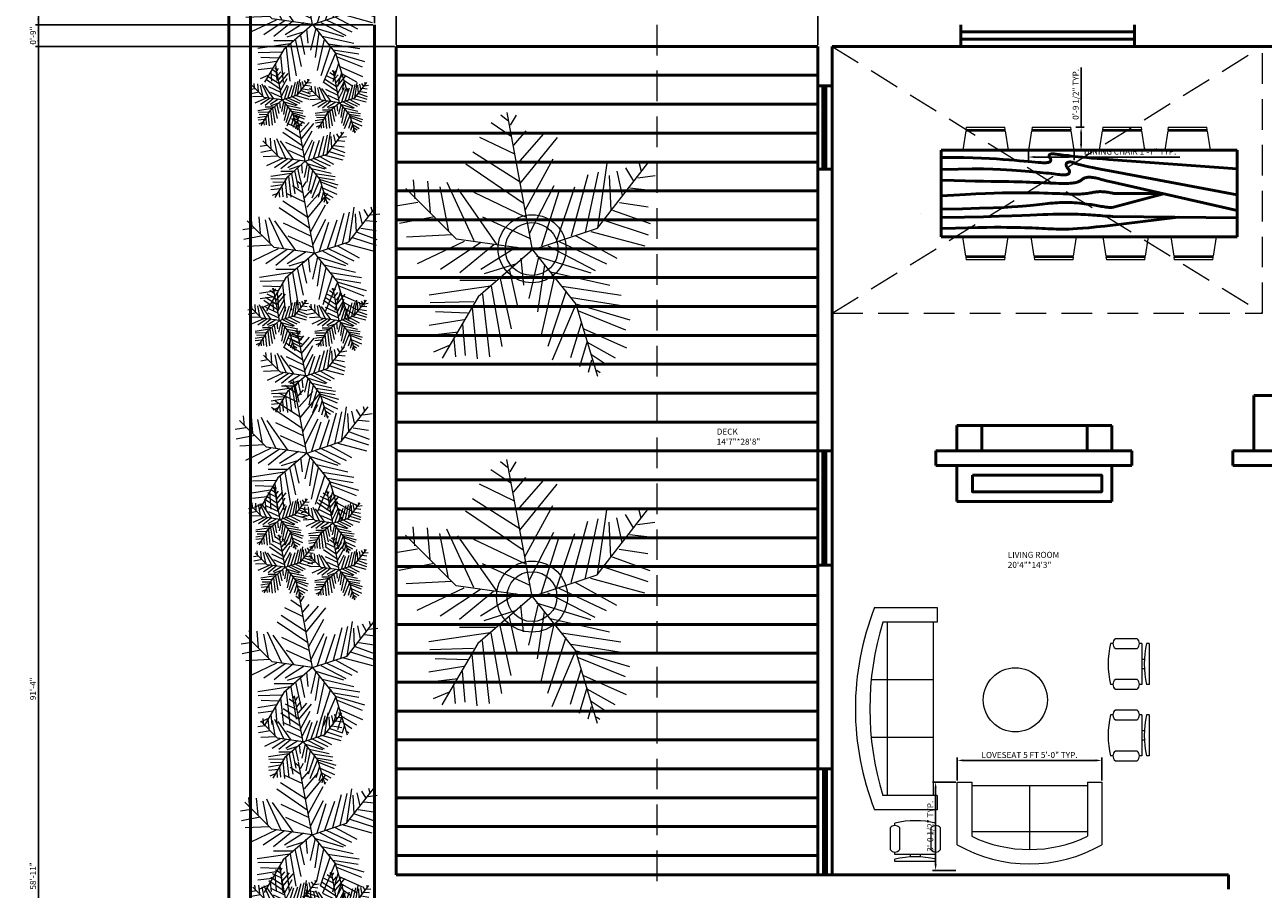
# Model space of a CAD drawing. Units: inches. Extents: x 5312 to 23584, y 2846 to 7447.
# Tile 2 of 12: x 8876 to 9390, y 3379 to 3738. Entities that reach past the tile are written whole.
import ezdxf

# ---------------------------------------------------------------- set-up
doc = ezdxf.new("R2010")
doc.units = ezdxf.units.IN
doc.linetypes.add('DASHED', pattern=[19.05, 12.7, -6.35])
for name, color, linetype, lineweight in [('A-ANNO-DIMS', 2, 'Continuous', 18), ('A-AREA-IDEN', 7, 'Continuous', 18), ('A-FLOR-OVHD', 8, 'DASHED', 18), ('A-FURN', 8, 'Continuous', 18), ('A-WALL', 7, 'Continuous', 50), ('L-PLNT', 82, 'Continuous', 13)]:
    doc.layers.add(name, color=color, linetype=linetype, lineweight=lineweight)
doc.styles.get("Standard").update_dxf_attribs({"font": 'arial.ttf'})
doc.dimstyles.new('ISO-25', dxfattribs={"dimtxt": 2.5, "dimasz": 2.5, "dimexe": 1.25, "dimexo": 0.625, "dimtad": 1, "dimlunit": 3, "dimtxsty": 'Standard', "dimcen": 2.5, "dimadec": 0, "dimazin": 0, "dimtfac": 1, "dimtmove": 0, "dimatfit": 3, "dimfxl": 1, "dimarcsym": 0})

# ---------------------------------------------------------------- blocks, each defined once
blk = doc.blocks.new('Sofa - Roundback 7 ft.')
for p, q in [((-12.00002, -32.4421), (-12.00003, -6.5971)), ((11.99997, -32.4421), (11.99998, -6.5971)), ((-36.000027, -34), (-36.000027, -11.4696)), ((-35.999844, -13.3819), (35.9998, -13.3819)), ((35.99998, -34), (35.99998, -11.4696)), ((-36.000027, -32.4421), (35.99998, -32.4421))]:
    blk.add_line(p, q)
for points in [[(-36.000027, -34), (-42.000027, -34), (-42.000027, -8)], [(41.99998, -8), (41.99998, -34), (35.99998, -34)]]:
    blk.add_lwpolyline(points)
for centre, radius, start, end in [((0, -114.25), 114.25, 68.43141, 111.5686), ((-0.00001, -127.1968), 121.1968, 72.72033, 107.2797)]:
    blk.add_arc(centre, radius, start, end)
blk = doc.blocks.new('Sofa - Roundback Loveseat 5 ft.')
for p, q in [((0, -32.44198), (0, -5.99998)), ((-24, -33.99998), (-24, -11.46958)), ((-23.9998, -13.38178), (23.99986, -13.38178)), ((24.00004, -33.99998), (24.00004, -11.46958)), ((-24, -32.44198), (24.00004, -32.44198))]:
    blk.add_line(p, q)
for points in [[(-24, -33.99998), (-30, -33.99998), (-30, -7.99998)], [(30.00004, -7.99998), (30.00004, -33.99998), (24.00004, -33.99998)]]:
    blk.add_lwpolyline(points)
for centre, radius, start, end in [((0, -60.24998), 60.24998, 60.13715, 119.8628), ((0, -61.38438), 55.38444, 64.32083, 115.6792)]:
    blk.add_arc(centre, radius, start, end)
blk = doc.blocks.new('Chair - Desk')
for p, q in [((-8.5, 0), (-8.5, -1)), ((-8.5, 0), (8.5, 0)), ((8.5, 0), (8.5, -1)), ((-10.5, -5), (-10.5, -14)), ((-8.5, -3), (-8.5, -4)), ((-8.5, -3), (8.5, -3)), ((-6.5, -14), (-6.5, -5)), ((-2, -3), (-2, -1.9355)), ((2, -1.9576), (2, -3)), ((6.5, -5), (6.5, -14)), ((8.5, -3), (8.5, -4)), ((10.5, -14), (10.5, -5)), ((-8.5, -15), (-8.5, -16)), ((8.5, -15), (8.5, -16))]:
    blk.add_line(p, q)
for centre, radius, start, end in [((-8.5, -6.5), 2.5, 36.8699, 143.1301), ((0, 34.625), 36.625, 256.5803, 283.4197), ((8.5, -6.5), 2.5, 36.8699, 143.1301), ((-8.5, -12.5), 2.5, 216.8699, 323.1301), ((8.5, -12.5), 2.5, 216.8699, 323.1301), ((0, 19.625), 36.625, 256.5803, 283.4197)]:
    blk.add_arc(centre, radius, start, end)
blk = doc.blocks.new('*U18')
for p, q in [((0, 0), (-10.5, 57)), ((-8.737, 47.138), (-17.069, 52.711)), ((-10.186, 53.64), (-13.084, 55.962)), ((-9.099, 51.782), (-6.563, 55.962)), ((-7.288, 39.707), (-21.778, 46.673)), ((-7.65, 43.423), (-2.578, 49.46)), ((-5.839, 35.992), (4.667, 48.067)), ((-5.114, 27.632), (10.463, 46.673)), ((-5.114, 28.097), (-24.676, 40.636)), ((-2.941, 16.486), (8.652, 37.85)), ((27, 9), (48, 36)), ((27.127, 9.056), (31.112, 35.992)), ((44.153, 36.456), (45.239, 32.741)), ((-3.665, 19.273), (-27.574, 35.527)), ((16.259, 5.805), (23.142, 31.348)), ((22.055, 7.198), (27.489, 32.277)), ((31.836, 30.883), (32.561, 16.486)), ((35.096, 32.741), (37.27, 22.524)), ((38.719, 34.134), (41.979, 28.561)), ((43.791, 29.954), (51.036, 30.883)), ((-48.585, 21.131), (-49.309, 29.026)), ((-43.513, 28.561), (-42.427, 15.558)), ((-38.442, 26.239), (-34.819, 7.663)), ((-35.544, 28.097), (-24.314, 3.947)), ((-1.129, 6.734), (9.014, 26.704)), ((10.101, 3.483), (17.708, 26.239)), ((40.53, 25.775), (48.862, 24.846)), ((-31.5, 4.5), (-52.5, 25.5)), ((-14.533, 2.09), (-30.834, 25.31)), ((-24.314, 23.917), (-2.941, 13.7)), ((3.942, 1.625), (11.187, 24.381)), ((-47.498, 19.737), (-55.83, 18.344)), ((33.285, 16.486), (48.862, 10.913)), ((36.183, 19.737), (48.137, 17.88)), ((-40.615, 13.7), (-55.105, 10.913)), ((-20.691, 13.7), (-1.129, 4.876)), ((29.662, 12.307), (48.137, 6.269)), ((-33.37, 6.269), (-52.207, 5.34)), ((0, 0), (27, 9)), ((18.07, 5.805), (35.096, -3.483)), ((24.229, 7.663), (46.688, 1.625)), ((-28.299, 3.483), (-47.86, -5.805)), ((-21.416, 3.018), (-38.079, -8.128)), ((0, 0), (-31.5, 4.5)), ((-15.982, 2.09), (-30.11, -9.521)), ((0, 0), (-22.5, -19.5)), ((-6.563, 1.161), (-21.416, -8.128)), ((0, 0), (18, -22.5)), ((6.478, 1.625), (26.04, -8.592)), ((11.187, 3.483), (30.749, -5.805)), ((-4.752, -3.483), (-3.665, -14.629)), ((2.493, -3.019), (-1.491, -20.202)), ((1.769, -2.555), (24.229, -9.521)), ((-6.563, -5.805), (-19.967, -9.985)), ((-9.461, -8.592), (-6.201, -23.453)), ((5.029, -6.27), (2.131, -25.775)), ((7.565, -9.056), (32.198, -14.629)), ((-17.431, -15.094), (-42.789, -18.809)), ((-15.257, -12.772), (-30.11, -12.772)), ((-17.069, -15.094), (-12.721, -40.172)), ((-13.446, -11.378), (-8.737, -32.741)), ((9.014, -11.378), (3.58, -35.992)), ((12.274, -15.094), (36.907, -18.809)), ((-22.5, -19.5), (-37.5, -45)), ((-20.691, -18.345), (-17.793, -44.352)), ((14.085, -16.951), (6.478, -40.172)), ((16.259, -19.738), (36.183, -22.989)), ((-24.314, -21.596), (-42.427, -22.06)), ((-25.038, -23.918), (-22.865, -45.281)), ((18.07, -22.524), (8.289, -45.745)), ((18, -22.5), (27, -52.5)), ((18.433, -22.524), (40.53, -29.026)), ((19.157, -25.311), (38.719, -33.206)), ((-28.299, -29.026), (-42.789, -31.348)), ((-26.849, -26.24), (-40.253, -25.775)), ((20.244, -30.419), (15.897, -44.816)), ((-30.834, -34.135), (-42.427, -35.528)), ((-29.023, -30.884), (-27.936, -43.887)), ((21.331, -32.741), (39.081, -40.636)), ((-34.457, -39.708), (-40.978, -42.494)), ((-32.646, -36.921), (-31.921, -44.352)), ((22.78, -37.85), (19.519, -48.532)), ((22.78, -38.314), (34.372, -44.816)), ((24.591, -45.745), (23.142, -50.854)), ((24.591, -43.423), (30.749, -47.603)), ((26.764, -49.925), (28.213, -50.854))]:
    blk.add_line(p, q)
blk = doc.blocks.new('CHAIR-DINING')
for p, q in [((1.25, 8), (0, 0)), ((1.25, 8), (17.72, 8)), ((1.48, 9.5), (1.33, 8.5)), ((17.64, 8.5), (1.33, 8.5)), ((1.48, 9.5), (17.48, 9.5)), ((17.64, 8.5), (17.48, 9.5)), ((18.97, 0), (17.72, 8))]:
    blk.add_line(p, q)
blk = doc.blocks.new('*D33')
at = {"layer": 'A-ANNO-DIMS', "color": 0, "lineweight": -2, "transparency": 16777216}
for p, q in [((9292.54, 3684.95), (9292.54, 3681.47)), ((9295.04, 3682.72), (9309.01, 3682.72)), ((9311.51, 3684.95), (9311.51, 3681.47)), ((9311.51, 3682.72), (9355.4, 3682.72))]:
    blk.add_line(p, q, dxfattribs=at)
at = {"layer": 'A-ANNO-DIMS', "color": 0, "transparency": 16777216}
for points in [[(9295.04, 3683.14), (9295.04, 3682.31), (9292.54, 3682.72)], [(9309.01, 3683.14), (9309.01, 3682.31), (9311.51, 3682.72)]]:
    blk.add_solid(points, dxfattribs=at)
at = {"layer": 'DEFPOINTS', "color": 0, "transparency": 16777216}
for p in [(9292.54, 3685.57), (9311.51, 3685.57), (9311.51, 3682.72)]:
    blk.add_point(p, dxfattribs=at)
at = {"layer": 'A-ANNO-DIMS', "color": 0, "transparency": 16777216, "insert": (9334.7, 3684.64), "char_height": 2.5, "attachment_point": 5}
blk.add_mtext('DINING CHAIR 1\'-7" TYP.', dxfattribs=at)
blk = doc.blocks.new('*D34')
at = {"layer": 'A-ANNO-DIMS', "color": 0, "lineweight": -2, "transparency": 16777216}
for p, q in [((9314.35, 3695.07), (9314.35, 3719.89)), ((9312.13, 3695.07), (9315.6, 3695.07)), ((9314.35, 3688.07), (9314.35, 3692.57)), ((9312.13, 3685.57), (9315.6, 3685.57))]:
    blk.add_line(p, q, dxfattribs=at)
at = {"layer": 'A-ANNO-DIMS', "color": 0, "transparency": 16777216}
for points in [[(9313.93, 3692.57), (9314.77, 3692.57), (9314.35, 3695.07)], [(9313.93, 3688.07), (9314.77, 3688.07), (9314.35, 3685.57)]]:
    blk.add_solid(points, dxfattribs=at)
at = {"layer": 'DEFPOINTS', "color": 0, "transparency": 16777216}
for p in [(9311.51, 3695.07), (9314.35, 3695.07), (9311.51, 3685.57)]:
    blk.add_point(p, dxfattribs=at)
at = {"layer": 'A-ANNO-DIMS', "color": 0, "transparency": 16777216, "insert": (9312.43, 3708.73), "char_height": 2.5, "attachment_point": 5, "rotation": 90}
blk.add_mtext('0\'-9 1/2" TYP.', dxfattribs=at)
blk = doc.blocks.new('*D37')
at = {"layer": 'A-ANNO-DIMS', "color": 0, "lineweight": -2, "transparency": 16777216}
for p, q in [((9262.95, 3423.77), (9262.95, 3433.4)), ((9320.45, 3432.15), (9265.45, 3432.15)), ((9322.95, 3423.77), (9322.95, 3433.4))]:
    blk.add_line(p, q, dxfattribs=at)
at = {"layer": 'A-ANNO-DIMS', "color": 0, "transparency": 16777216}
for points in [[(9265.45, 3432.57), (9265.45, 3431.73), (9262.95, 3432.15)], [(9320.45, 3432.57), (9320.45, 3431.73), (9322.95, 3432.15)]]:
    blk.add_solid(points, dxfattribs=at)
at = {"layer": 'DEFPOINTS', "color": 0, "transparency": 16777216}
for p in [(9262.95, 3432.15), (9262.95, 3423.15), (9322.95, 3423.15)]:
    blk.add_point(p, dxfattribs=at)
at = {"layer": 'A-ANNO-DIMS', "color": 0, "transparency": 16777216, "insert": (9292.95, 3434.07), "char_height": 2.5, "attachment_point": 5}
blk.add_mtext('LOVESEAT 5 FT 5\'-0" TYP.', dxfattribs=at)
blk = doc.blocks.new('*D38')
at = {"layer": 'A-ANNO-DIMS', "color": 0, "lineweight": -2, "transparency": 16777216}
for p, q in [((9262.32, 3423.15), (9252.7, 3423.15)), ((9253.95, 3420.65), (9253.95, 3388.98)), ((9262.32, 3386.48), (9252.7, 3386.48))]:
    blk.add_line(p, q, dxfattribs=at)
at = {"layer": 'A-ANNO-DIMS', "color": 0, "transparency": 16777216}
for points in [[(9253.53, 3420.65), (9254.37, 3420.65), (9253.95, 3423.15)], [(9253.53, 3388.98), (9254.37, 3388.98), (9253.95, 3386.48)]]:
    blk.add_solid(points, dxfattribs=at)
at = {"layer": 'DEFPOINTS', "color": 0, "transparency": 16777216}
for p in [(9262.95, 3423.15), (9253.95, 3386.48), (9262.95, 3386.48)]:
    blk.add_point(p, dxfattribs=at)
at = {"layer": 'A-ANNO-DIMS', "color": 0, "transparency": 16777216, "insert": (9252.03, 3404.82), "char_height": 2.5, "attachment_point": 5, "rotation": 90}
blk.add_mtext('3\'-0 1/2" TYP.', dxfattribs=at)
blk = doc.blocks.new('*D47')
at = {"layer": 'A-ANNO-DIMS', "color": 0, "lineweight": -2, "transparency": 16777216}
for p, q in [((8959.95, 4009.84), (8880.22, 4009.84)), ((8881.47, 4007.34), (8881.47, 2916.4)), ((8952.19, 2913.9), (8880.22, 2913.9))]:
    blk.add_line(p, q, dxfattribs=at)
at = {"layer": 'A-ANNO-DIMS', "color": 0, "transparency": 16777216}
for points in [[(8881.05, 4007.34), (8881.89, 4007.34), (8881.47, 4009.84)], [(8881.05, 2916.4), (8881.89, 2916.4), (8881.47, 2913.9)]]:
    blk.add_solid(points, dxfattribs=at)
at = {"layer": 'DEFPOINTS', "color": 0, "transparency": 16777216}
for p in [(8960.57, 4009.84), (8881.47, 2913.9), (8952.82, 2913.9)]:
    blk.add_point(p, dxfattribs=at)
at = {"layer": 'A-ANNO-DIMS', "color": 0, "transparency": 16777216, "insert": (8879.57, 3461.87), "char_height": 2.5, "attachment_point": 5, "rotation": 90}
blk.add_mtext('91\'-4"', dxfattribs=at)
blk = doc.blocks.new('*D48')
at = {"layer": 'A-ANNO-DIMS', "color": 0, "lineweight": -2, "transparency": 16777216}
for p, q in [((9021.01, 3738.27), (9021.01, 4212.68)), ((9023.51, 4211.43), (9652.51, 4211.43)), ((9655.01, 3738.27), (9655.01, 4212.68))]:
    blk.add_line(p, q, dxfattribs=at)
at = {"layer": 'A-ANNO-DIMS', "color": 0, "transparency": 16777216}
for points in [[(9023.51, 4211.85), (9023.51, 4211.01), (9021.01, 4211.43)], [(9652.51, 4211.85), (9652.51, 4211.01), (9655.01, 4211.43)]]:
    blk.add_solid(points, dxfattribs=at)
at = {"layer": 'DEFPOINTS', "color": 0, "transparency": 16777216}
for p in [(9655.01, 4211.43), (9021.01, 3737.65), (9655.01, 3737.65)]:
    blk.add_point(p, dxfattribs=at)
at = {"layer": 'A-ANNO-DIMS', "color": 0, "transparency": 16777216, "insert": (9338.01, 4213.33), "char_height": 2.5, "attachment_point": 5}
blk.add_mtext('52\'-10"', dxfattribs=at)
blk = doc.blocks.new('*D51')
at = {"layer": 'A-ANNO-DIMS', "color": 0, "lineweight": -2, "transparency": 16777216}
for p, q in [((9020.38, 3894.91), (8880.22, 3894.91)), ((8881.47, 3892.41), (8881.47, 3740.15)), ((9020.38, 3737.65), (8880.22, 3737.65))]:
    blk.add_line(p, q, dxfattribs=at)
at = {"layer": 'A-ANNO-DIMS', "color": 0, "transparency": 16777216}
for points in [[(8881.05, 3892.41), (8881.89, 3892.41), (8881.47, 3894.91)], [(8881.05, 3740.15), (8881.89, 3740.15), (8881.47, 3737.65)]]:
    blk.add_solid(points, dxfattribs=at)
at = {"layer": 'DEFPOINTS', "color": 0, "transparency": 16777216}
for p in [(9021.01, 3894.91), (8881.47, 3737.65), (9021.01, 3737.65)]:
    blk.add_point(p, dxfattribs=at)
at = {"layer": 'A-ANNO-DIMS', "color": 0, "transparency": 16777216, "insert": (8879.55, 3816.28), "char_height": 2.5, "attachment_point": 5, "rotation": 90}
blk.add_mtext('13\'-1 1/2"', dxfattribs=at)
blk = doc.blocks.new('*D52')
at = {"layer": 'A-ANNO-DIMS', "color": 0, "lineweight": -2, "transparency": 16777216}
for p, q in [((9020.38, 3737.65), (8880.22, 3737.65)), ((8881.47, 3735.15), (8881.47, 3033.15)), ((9020.38, 3030.65), (8880.22, 3030.65))]:
    blk.add_line(p, q, dxfattribs=at)
at = {"layer": 'A-ANNO-DIMS', "color": 0, "transparency": 16777216}
for points in [[(8881.05, 3735.15), (8881.89, 3735.15), (8881.47, 3737.65)], [(8881.05, 3033.15), (8881.89, 3033.15), (8881.47, 3030.65)]]:
    blk.add_solid(points, dxfattribs=at)
at = {"layer": 'DEFPOINTS', "color": 0, "transparency": 16777216}
for p in [(9021.01, 3737.65), (8881.47, 3030.65), (9021.01, 3030.65)]:
    blk.add_point(p, dxfattribs=at)
at = {"layer": 'A-ANNO-DIMS', "color": 0, "transparency": 16777216, "insert": (8879.57, 3384.15), "char_height": 2.5, "attachment_point": 5, "rotation": 90}
blk.add_mtext('58\'-11"', dxfattribs=at)
blk = doc.blocks.new('*D54')
at = {"layer": 'A-ANNO-DIMS', "color": 0, "lineweight": -2, "transparency": 16777216}
for p, q in [((9030.01, 3729.27), (9030.01, 4212.68)), ((9032.51, 4211.43), (9202.51, 4211.43)), ((9205.01, 3729.27), (9205.01, 4212.68))]:
    blk.add_line(p, q, dxfattribs=at)
at = {"layer": 'A-ANNO-DIMS', "color": 0, "transparency": 16777216}
for points in [[(9032.51, 4211.85), (9032.51, 4211.01), (9030.01, 4211.43)], [(9202.51, 4211.85), (9202.51, 4211.01), (9205.01, 4211.43)]]:
    blk.add_solid(points, dxfattribs=at)
at = {"layer": 'DEFPOINTS', "color": 0, "transparency": 16777216}
for p in [(9205.01, 4211.43), (9030.01, 3728.65), (9205.01, 3728.65)]:
    blk.add_point(p, dxfattribs=at)
at = {"layer": 'A-ANNO-DIMS', "color": 0, "transparency": 16777216, "insert": (9117.51, 4213.31), "char_height": 2.5, "attachment_point": 5}
blk.add_mtext('14\'-7"', dxfattribs=at)
blk = doc.blocks.new('*D55')
at = {"layer": 'A-ANNO-DIMS', "color": 0, "lineweight": -2, "transparency": 16777216}
for p, q in [((9205.01, 3729.27), (9205.01, 4212.68)), ((9207.51, 4211.43), (9531.51, 4211.43)), ((9534.01, 3705.2), (9534.01, 4212.68))]:
    blk.add_line(p, q, dxfattribs=at)
at = {"layer": 'A-ANNO-DIMS', "color": 0, "transparency": 16777216}
for points in [[(9207.51, 4211.85), (9207.51, 4211.01), (9205.01, 4211.43)], [(9531.51, 4211.85), (9531.51, 4211.01), (9534.01, 4211.43)]]:
    blk.add_solid(points, dxfattribs=at)
at = {"layer": 'DEFPOINTS', "color": 0, "transparency": 16777216}
for p in [(9534.01, 4211.43), (9205.01, 3728.65), (9534.01, 3704.57)]:
    blk.add_point(p, dxfattribs=at)
at = {"layer": 'A-ANNO-DIMS', "color": 0, "transparency": 16777216, "insert": (9369.51, 4213.33), "char_height": 2.5, "attachment_point": 5}
blk.add_mtext('27\'-5"', dxfattribs=at)
blk = doc.blocks.new('*D58')
at = {"layer": 'A-ANNO-DIMS', "color": 0, "lineweight": -2, "transparency": 16777216}
for p, q in [((9020.38, 3737.65), (8880.22, 3737.65)), ((8881.47, 3735.15), (8881.47, 3731.15)), ((9029.38, 3728.65), (8880.22, 3728.65))]:
    blk.add_line(p, q, dxfattribs=at)
at = {"layer": 'A-ANNO-DIMS', "color": 0, "transparency": 16777216}
for points in [[(8881.05, 3735.15), (8881.89, 3735.15), (8881.47, 3737.65)], [(8881.05, 3731.15), (8881.89, 3731.15), (8881.47, 3728.65)]]:
    blk.add_solid(points, dxfattribs=at)
at = {"layer": 'DEFPOINTS', "color": 0, "transparency": 16777216}
for p in [(9021.01, 3737.65), (8881.47, 3728.65), (9030.01, 3728.65)]:
    blk.add_point(p, dxfattribs=at)
at = {"layer": 'A-ANNO-DIMS', "color": 0, "transparency": 16777216, "insert": (8879.57, 3733.15), "char_height": 2.5, "attachment_point": 5, "rotation": 90}
blk.add_mtext('0\'-9"', dxfattribs=at)

msp = doc.modelspace()

# ---------------------------------------------------------------- linework, layer by layer
at = {"layer": 'A-FLOR-OVHD'}
for p, q in [((9138.223, 3737.646), (9138.223, 3378.646)), ((9211.009, 3728.646), (9389.615, 3617.875)), ((9211.009, 3617.875), (9389.615, 3728.646)), ((9389.615, 3617.875), (9389.615, 3728.646)), ((9211.009, 3617.875), (9389.615, 3617.875))]:
    msp.add_line(p, q, dxfattribs=at)
at = {"layer": 'A-FURN'}
for centre, radius in [((9086.443, 3644.646), 14.113), ((9086.261, 3644.5), 10.979), ((9086.399, 3500.16), 14.745), ((9086.399, 3500.16), 10.358), ((9287.056, 3457.302), 13.311)]:
    msp.add_circle(centre, radius, dxfattribs=at)
at = {"layer": 'A-WALL'}
for p, q in [((8960.573, 4009.837), (8960.573, 3030.646)), ((8969.573, 4000.837), (8969.573, 3030.646)), ((9021.009, 3737.646), (9021.009, 3030.646)), ((9264.453, 3728.646), (9264.453, 3737.646)), ((9264.453, 3734.646), (9336.453, 3734.646)), ((9336.453, 3737.646), (9336.453, 3728.646)), ((9030.009, 3728.646), (9030.009, 3384.646)), ((9205.009, 3728.646), (9030.009, 3728.646)), ((9205.009, 3728.646), (9205.009, 3384.646)), ((9211.009, 3728.646), (9211.009, 3384.646)), ((9534.009, 3728.646), (9211.009, 3728.646)), ((9336.453, 3731.646), (9264.453, 3731.646)), ((9336.453, 3728.646), (9264.453, 3728.646)), ((9030.009, 3716.646), (9205.009, 3716.646)), ((9205.009, 3712.35), (9205.009, 3712.35)), ((9205.009, 3712.35), (9211.009, 3712.35)), ((9207.135, 3712.35), (9207.135, 3712.181)), ((9207.135, 3712.181), (9207.135, 3677.701)), ((9208.364, 3712.35), (9208.364, 3677.701)), ((9030.009, 3704.646), (9205.009, 3704.646)), ((9030.009, 3692.646), (9205.009, 3692.646)), ((9328.311, 3685.573), (9256.311, 3685.573)), ((9256.311, 3685.573), (9256.311, 3649.573)), ((9328.311, 3685.573), (9379.173, 3685.573)), ((9379.173, 3685.573), (9379.173, 3649.573)), ((9030.009, 3680.646), (9205.009, 3680.646)), ((9205.009, 3677.701), (9211.009, 3677.701)), ((9256.311, 3677.057), (9256.314, 3677.058)), ((9328.311, 3677.057), (9328.309, 3677.058)), ((9030.009, 3668.646), (9205.009, 3668.646)), ((9030.009, 3656.646), (9205.009, 3656.646)), ((9247.811, 3659.414), (9247.811, 3659.417)), ((9256.314, 3658.088), (9256.311, 3658.088)), ((9328.309, 3658.088), (9328.311, 3658.088)), ((9336.811, 3659.414), (9336.811, 3659.417)), ((9256.311, 3649.573), (9328.311, 3649.573)), ((9379.173, 3649.573), (9328.311, 3649.573)), ((9030.009, 3644.646), (9205.009, 3644.646)), ((9030.009, 3632.646), (9205.009, 3632.646)), ((9030.009, 3620.646), (9205.009, 3620.646)), ((9030.009, 3608.646), (9205.009, 3608.646)), ((9030.009, 3596.646), (9205.009, 3596.646)), ((9030.009, 3584.646), (9205.009, 3584.646)), ((9386.03, 3560.646), (9386.03, 3583.618)), ((9386.03, 3583.618), (9412.168, 3583.618)), ((9030.009, 3572.646), (9205.009, 3572.646)), ((9262.818, 3560.646), (9262.818, 3571.256)), ((9262.818, 3571.256), (9273.074, 3571.256)), ((9273.074, 3571.256), (9273.074, 3560.646)), ((9273.074, 3571.256), (9273.074, 3571.256)), ((9273.074, 3571.256), (9316.902, 3571.256)), ((9327.153, 3571.256), (9316.902, 3571.256)), ((9316.902, 3571.256), (9316.902, 3560.646)), ((9327.153, 3560.646), (9327.153, 3571.256)), ((9030.009, 3560.646), (9205.009, 3560.646)), ((9211.009, 3560.646), (9205.009, 3560.646)), ((9207.089, 3560.646), (9207.089, 3513.246)), ((9208.383, 3560.646), (9208.383, 3513.252)), ((9254.065, 3560.646), (9254.065, 3554.646)), ((9335.425, 3560.646), (9254.065, 3560.646)), ((9335.425, 3560.646), (9335.425, 3554.646)), ((9534.009, 3560.646), (9377.388, 3560.646)), ((9377.388, 3560.646), (9377.388, 3554.646)), ((9386.03, 3560.646), (9386.03, 3560.646)), ((9335.425, 3554.646), (9254.065, 3554.646)), ((9262.818, 3554.646), (9262.818, 3539.628)), ((9327.153, 3539.628), (9327.153, 3554.646)), ((9540.009, 3554.646), (9377.388, 3554.646)), ((9030.009, 3548.646), (9205.009, 3548.646)), ((9262.818, 3539.628), (9327.153, 3539.628)), ((9030.009, 3536.646), (9205.009, 3536.646)), ((9030.009, 3524.646), (9205.009, 3524.646)), ((9030.009, 3512.646), (9205.009, 3512.646)), ((9205.009, 3513.252), (9205.009, 3513.252)), ((9205.009, 3513.252), (9211.009, 3513.252)), ((9030.009, 3500.646), (9205.009, 3500.646)), ((9030.009, 3488.646), (9205.009, 3488.646)), ((9030.009, 3476.646), (9205.009, 3476.646)), ((9030.009, 3464.646), (9205.009, 3464.646)), ((9030.009, 3452.646), (9205.009, 3452.646)), ((9030.009, 3440.646), (9205.009, 3440.646)), ((9030.009, 3428.646), (9205.009, 3428.646)), ((9205.009, 3428.646), (9211.009, 3428.646)), ((9207.407, 3428.646), (9207.407, 3384.646)), ((9208.666, 3428.646), (9208.666, 3384.646)), ((9030.009, 3416.646), (9205.009, 3416.646)), ((9030.009, 3404.646), (9205.009, 3404.646)), ((9030.009, 3392.646), (9205.009, 3392.646)), ((9211.009, 3384.646), (9030.009, 3384.646)), ((9211.009, 3384.646), (9375.565, 3384.646)), ((9375.565, 3378.646), (9375.565, 3384.646))]:
    msp.add_line(p, q, dxfattribs=at)
for points in [[(9256.311, 3682.573), (9261.134, 3682.55), (9265.504, 3682.487), (9269.458, 3682.388), (9273.035, 3682.26), (9276.275, 3682.109), (9279.216, 3681.94), (9281.896, 3681.759), (9284.353, 3681.573), (9286.621, 3681.386), (9288.708, 3681.203), (9290.616, 3681.028), (9292.348, 3680.864), (9293.906, 3680.717), (9295.293, 3680.588), (9296.51, 3680.484), (9297.561, 3680.406), (9298.451, 3680.359), (9299.192, 3680.341), (9299.8, 3680.35), (9300.291, 3680.385), (9300.68, 3680.444), (9300.983, 3680.523), (9301.216, 3680.623), (9301.395, 3680.739), (9301.532, 3680.872), (9301.633, 3681.017), (9301.701, 3681.172), (9301.739, 3681.333), (9301.749, 3681.499), (9301.735, 3681.665), (9301.699, 3681.83), (9301.645, 3681.989), (9301.575, 3682.142), (9301.495, 3682.288), (9301.409, 3682.427), (9301.322, 3682.562), (9301.239, 3682.693), (9301.164, 3682.821), (9301.104, 3682.948), (9301.061, 3683.073), (9301.042, 3683.197), (9301.046, 3683.32), (9301.073, 3683.439), (9301.124, 3683.552), (9301.198, 3683.657), (9301.296, 3683.752), (9301.417, 3683.836), (9301.561, 3683.906), (9301.73, 3683.961), (9301.929, 3684), (9302.162, 3684.023), (9302.436, 3684.031), (9302.758, 3684.023), (9303.132, 3684), (9303.564, 3683.961), (9304.061, 3683.906), (9304.63, 3683.836), (9305.281, 3683.751), (9306.027, 3683.653), (9306.879, 3683.542), (9307.851, 3683.419), (9308.954, 3683.285), (9310.201, 3683.142), (9311.603, 3682.989), (9313.17, 3682.829), (9314.899, 3682.663), (9316.784, 3682.49), (9318.817, 3682.312), (9320.992, 3682.131), (9323.304, 3681.946), (9325.746, 3681.76), (9379.173, 3677.859)], [(9256.311, 3677.573), (9263.335, 3677.716), (9269.139, 3677.777), (9273.887, 3677.771), (9277.744, 3677.708), (9280.872, 3677.603), (9283.434, 3677.467), (9285.596, 3677.314), (9287.52, 3677.156), (9289.342, 3677.004), (9291.087, 3676.858), (9292.753, 3676.718), (9294.337, 3676.583), (9295.838, 3676.452), (9297.252, 3676.324), (9298.577, 3676.198), (9299.811, 3676.073), (9300.953, 3675.948), (9302.003, 3675.827), (9302.965, 3675.711), (9303.843, 3675.604), (9304.638, 3675.509), (9305.354, 3675.428), (9305.995, 3675.365), (9306.561, 3675.323), (9307.059, 3675.303), (9307.491, 3675.306), (9307.865, 3675.33), (9308.186, 3675.375), (9308.461, 3675.439), (9308.694, 3675.522), (9308.893, 3675.622), (9309.061, 3675.739), (9309.206, 3675.872), (9309.326, 3676.018), (9309.42, 3676.176), (9309.489, 3676.344), (9309.529, 3676.519), (9309.542, 3676.7), (9309.525, 3676.886), (9309.478, 3677.073), (9309.401, 3677.26), (9309.298, 3677.448), (9309.176, 3677.635), (9309.041, 3677.823), (9308.897, 3678.01), (9308.752, 3678.198), (9308.61, 3678.385), (9308.478, 3678.573), (9308.361, 3678.76), (9308.263, 3678.946), (9308.187, 3679.131), (9308.134, 3679.312), (9308.109, 3679.49), (9308.115, 3679.663), (9308.153, 3679.829), (9308.228, 3679.989), (9308.341, 3680.141), (9308.49, 3680.281), (9308.672, 3680.405), (9308.884, 3680.51), (9309.124, 3680.592), (9309.388, 3680.646), (9309.674, 3680.668), (9309.978, 3680.656), (9310.301, 3680.606), (9310.653, 3680.52), (9311.05, 3680.402), (9311.504, 3680.255), (9312.031, 3680.083), (9312.644, 3679.889), (9313.358, 3679.676), (9314.186, 3679.448), (9315.147, 3679.206), (9316.27, 3678.946), (9317.59, 3678.659), (9319.14, 3678.338), (9320.953, 3677.977), (9323.063, 3677.567), (9325.505, 3677.101), (9379.173, 3666.994)], [(9256.311, 3673.073), (9261.596, 3672.908), (9266.242, 3672.782), (9270.317, 3672.69), (9273.884, 3672.625), (9277.011, 3672.579), (9279.761, 3672.545), (9282.2, 3672.518), (9284.395, 3672.489), (9286.402, 3672.454), (9288.253, 3672.413), (9289.969, 3672.365), (9291.572, 3672.312), (9293.085, 3672.256), (9294.531, 3672.196), (9295.933, 3672.135), (9297.311, 3672.073), (9298.684, 3672.011), (9300.046, 3671.95), (9301.384, 3671.894), (9302.686, 3671.844), (9303.942, 3671.801), (9305.14, 3671.768), (9306.267, 3671.747), (9307.311, 3671.739), (9308.265, 3671.747), (9309.13, 3671.771), (9309.912, 3671.81), (9310.614, 3671.864), (9311.241, 3671.935), (9311.8, 3672.021), (9312.294, 3672.122), (9312.728, 3672.239), (9313.108, 3672.372), (9313.442, 3672.517), (9313.736, 3672.672), (9313.999, 3672.833), (9314.239, 3672.999), (9314.463, 3673.165), (9314.679, 3673.33), (9314.895, 3673.489), (9315.118, 3673.641), (9315.352, 3673.784), (9315.599, 3673.914), (9315.864, 3674.031), (9316.147, 3674.132), (9316.453, 3674.216), (9316.785, 3674.28), (9317.145, 3674.323), (9317.535, 3674.342), (9317.953, 3674.34), (9318.397, 3674.315), (9318.864, 3674.271), (9319.349, 3674.206), (9319.852, 3674.124), (9320.368, 3674.023), (9320.895, 3673.906), (9321.436, 3673.773), (9322.019, 3673.62), (9322.678, 3673.443), (9323.447, 3673.239), (9324.361, 3673.004), (9325.453, 3672.734), (9326.759, 3672.425), (9379.173, 3660.534)], [(9256.311, 3666.573), (9261.52, 3666.914), (9266.292, 3667.191), (9270.66, 3667.41), (9274.655, 3667.578), (9278.311, 3667.701), (9281.659, 3667.786), (9284.732, 3667.838), (9287.561, 3667.864), (9290.177, 3667.871), (9292.599, 3667.86), (9294.843, 3667.834), (9296.926, 3667.797), (9298.864, 3667.749), (9300.675, 3667.695), (9302.374, 3667.635), (9303.978, 3667.573), (9305.501, 3667.511), (9306.946, 3667.452), (9308.31, 3667.398), (9309.593, 3667.354), (9310.794, 3667.321), (9311.912, 3667.303), (9312.946, 3667.303), (9313.895, 3667.323), (9314.76, 3667.365), (9315.547, 3667.427), (9316.266, 3667.504), (9316.926, 3667.594), (9317.535, 3667.691), (9318.102, 3667.792), (9318.636, 3667.892), (9319.145, 3667.989), (9319.638, 3668.079), (9320.121, 3668.159), (9320.601, 3668.227), (9321.082, 3668.281), (9321.572, 3668.32), (9322.074, 3668.341), (9322.597, 3668.343), (9323.145, 3668.323), (9323.72, 3668.281), (9324.311, 3668.22), (9324.9, 3668.146), (9325.473, 3668.062), (9326.012, 3667.975), (9326.502, 3667.889), (9326.927, 3667.809), (9327.27, 3667.739), (9327.521, 3667.684), (9327.696, 3667.643), (9327.815, 3667.613), (9327.9, 3667.594), (9327.971, 3667.582), (9328.049, 3667.575), (9328.156, 3667.573), (9348.328, 3667.532)], [(9256.311, 3661.073), (9265.127, 3661.26), (9272.227, 3661.446), (9277.842, 3661.631), (9282.202, 3661.812), (9285.536, 3661.99), (9288.075, 3662.163), (9290.049, 3662.329), (9291.686, 3662.489), (9293.182, 3662.642), (9294.583, 3662.786), (9295.899, 3662.923), (9297.14, 3663.052), (9298.316, 3663.173), (9299.438, 3663.286), (9300.517, 3663.392), (9301.561, 3663.489), (9302.582, 3663.579), (9303.585, 3663.659), (9304.576, 3663.727), (9305.561, 3663.781), (9306.547, 3663.82), (9307.538, 3663.841), (9308.541, 3663.843), (9309.561, 3663.823), (9310.603, 3663.78), (9311.657, 3663.717), (9312.712, 3663.637), (9313.759, 3663.542), (9314.787, 3663.435), (9315.784, 3663.319), (9316.74, 3663.197), (9317.645, 3663.073), (9318.49, 3662.948), (9319.281, 3662.823), (9320.026, 3662.7), (9320.733, 3662.578), (9321.411, 3662.458), (9322.069, 3662.34), (9322.713, 3662.226), (9323.353, 3662.114), (9323.995, 3662.008), (9324.638, 3661.915), (9325.277, 3661.841), (9325.91, 3661.797), (9326.534, 3661.789), (9327.144, 3661.827), (9327.738, 3661.919), (9348.519, 3667.488)], [(9256.311, 3657.573), (9265.909, 3657.76), (9273.844, 3657.944), (9280.328, 3658.122), (9285.572, 3658.292), (9289.789, 3658.449), (9293.19, 3658.592), (9295.988, 3658.718), (9298.395, 3658.823), (9300.588, 3658.905), (9302.614, 3658.966), (9304.483, 3659.007), (9306.207, 3659.031), (9307.799, 3659.039), (9309.27, 3659.034), (9310.631, 3659.016), (9311.895, 3658.989), (9313.073, 3658.954), (9314.18, 3658.912), (9315.23, 3658.863), (9316.239, 3658.807), (9317.22, 3658.746), (9318.188, 3658.679), (9319.158, 3658.607), (9320.145, 3658.531), (9321.159, 3658.452), (9322.194, 3658.372), (9323.241, 3658.295), (9324.291, 3658.224), (9325.332, 3658.163), (9326.356, 3658.115), (9327.352, 3658.084), (9379.173, 3657.482)], [(9256.311, 3653.073), (9262.223, 3653.238), (9267.278, 3653.361), (9271.58, 3653.446), (9275.233, 3653.5), (9278.341, 3653.526), (9281.009, 3653.53), (9283.339, 3653.516), (9285.436, 3653.489), (9287.389, 3653.454), (9289.221, 3653.413), (9290.941, 3653.365), (9292.556, 3653.312), (9294.076, 3653.256), (9295.509, 3653.196), (9296.862, 3653.135), (9298.145, 3653.073), (9299.367, 3653.011), (9300.546, 3652.951), (9301.704, 3652.896), (9302.858, 3652.849), (9304.031, 3652.811), (9305.24, 3652.786), (9306.508, 3652.775), (9307.853, 3652.781), (9309.305, 3652.809), (9310.927, 3652.868), (9312.792, 3652.971), (9314.973, 3653.13), (9317.543, 3653.358), (9320.574, 3653.666), (9324.139, 3654.067), (9354.65, 3657.767)]]:
    msp.add_lwpolyline(points, dxfattribs=at)
msp.add_lwpolyline([(9269.237, 3550.576), (9322.915, 3550.576), (9322.915, 3543.688), (9269.237, 3543.688)], close=True, dxfattribs=at)

# ---------------------------------------------------------------- block references
at = {"layer": 'A-FURN'}
for p in [(9265.189, 3685.57), (9292.537, 3685.57), (9321.877, 3685.572)]:
    msp.add_blockref('CHAIR-DINING', p, dxfattribs=at)
for name, p, rotation in [('CHAIR-DINING', (9349.04, 3685.572), 359.9996510728321), ('CHAIR-DINING', (9284.135, 3649.574), 180.0056718243519), ('CHAIR-DINING', (9312.498, 3649.574), 180.0056718243519), ('CHAIR-DINING', (9342.321, 3649.577), 180.0056718243519), ('CHAIR-DINING', (9370.506, 3649.577), 180.0056718243519), ('Sofa - Roundback 7 ft.', (9220.632, 3453.606), 90), ('Chair - Desk', (9342.563, 3472.185), 270), ('Chair - Desk', (9342.563, 3442.524), 270), ('Sofa - Roundback Loveseat 5 ft.', (9292.95, 3389.149), 180), ('Chair - Desk', (9245.528, 3390.101), 180)]:
    msp.add_blockref(name, p, dxfattribs=dict(at, rotation=rotation))
at = {"layer": 'L-PLNT'}
for p, xscale, yscale, zscale in [((8995.269, 3737.769), 0.5312656759052281, 0.5312656759052281, 0.5312656759052281), ((8982.699, 3706.404), 0.2364091890538949, 0.2364091890538949, 0.2364091890538949), ((9006.48, 3705.226), 0.2364091890538949, 0.2364091890538949, 0.2364091890538949), ((8992.261, 3680.943), 0.3351400291328743, 0.3351400291328743, 0.3351400291328743), ((8996.066, 3642.733), 0.5312656759052281, 0.5312656759052281, 0.5312656759052281), ((8981.566, 3614.768), 0.2364091890538949, 0.2364091890538949, 0.2364091890538949), ((9006.334, 3614.727), 0.2364091890538949, 0.2364091890538949, 0.2364091890538949), ((8992.488, 3591.833), 0.3351400291328743, 0.3351400291328743, 0.3351400291328743), ((8992.881, 3559.8), 0.5312656759052281, 0.5312656759052281, 0.5312656759052281), ((8981.834, 3532.256), 0.2364091890538949, 0.2364091890538949, 0.2364091890538949), ((9003.779, 3530.649), 0.2364091890538949, 0.2364091890538949, 0.2364091890538949), ((8983.939, 3512.328), 0.2364091890538949, 0.2364091890538949, 0.2364091890538949), ((9006.316, 3511.221), 0.2364091890538949, 0.2364091890538949, 0.2364091890538949), ((8995.314, 3470.672), 0.5312656759052281, 0.5312656759052281, 0.5312656759052281), ((8991.349, 3439.877), 0.3351400291328743, 0.3351400291328743, 0.3351400291328743), ((8995.071, 3401.266), 0.5312656759052281, 0.5312656759052281, 0.5312656759052281), ((8984.482, 3372.686), 0.2657412829208717, 0.2657412829208717, 0.2657412829208717), ((9005.902, 3370.648), 0.2657412829208717, 0.2657412829208717, 0.2657412829208717)]:
    msp.add_blockref('*U18', p, dxfattribs=dict(at, xscale=xscale, yscale=yscale, zscale=zscale))
for p in [(9086.533, 3644.16), (9086.399, 3500.16)]:
    msp.add_blockref('*U18', p, dxfattribs=at)

# ---------------------------------------------------------------- texts
at = {"layer": 'A-AREA-IDEN', "char_height": 2.5, "attachment_point": 1}
for s, width, insert in [('DECK\\P\\pxt6;14\'7"*28\'8"', 41.37353, (9163.081, 3569.927)), ('LIVING ROOM\\P20\'4"*14\'3"', 72.68615, (9283.917, 3518.763))]:
    msp.add_mtext_dynamic_manual_height_columns(s, width=width, gutter_width=12.5, heights=[0], dxfattribs=dict(at, insert=insert))

# ---------------------------------------------------------------- dimensions: what is measured, and where the dimension line sits
at = {"layer": 'A-ANNO-DIMS'}
for base, p1, p2, picture, middle in [((9655.009, 4211.429), (9021.009, 3737.646), (9655.009, 3737.646), '*D48', (9338.009, 4213.33)), ((9205.009, 4211.429), (9030.009, 3728.646), (9205.009, 3728.646), '*D54', (9117.509, 4213.309)), ((9534.009, 4211.429), (9205.009, 3728.646), (9534.009, 3704.571), '*D55', (9369.509, 4213.33))]:
    dim = msp.add_linear_dim(base=base, p1=p1, p2=p2, dimstyle='ISO-25', override={"dimdec": 1, "dimlfac": 1, "dimrnd": 0, "dimzin": 1, "dimdsep": 46, "dimlunit": 4, "dimfrac": 2}, dxfattribs=at)
    dim.commit()
    dim.dimension.update_dxf_attribs({"geometry": picture, "text_midpoint": middle})
for base, p1, p2, picture, middle in [((8881.47, 2913.9), (8960.573, 4009.837), (8952.82, 2913.9), '*D47', (8879.569, 3461.869)), ((8881.47, 3737.646), (9021.009, 3894.906), (9021.009, 3737.646), '*D51', (8879.552, 3816.276)), ((8881.47, 3030.646), (9021.009, 3737.646), (9021.009, 3030.646), '*D52', (8879.569, 3384.146)), ((8881.47, 3728.646), (9021.009, 3737.646), (9030.009, 3728.646), '*D58', (8879.569, 3733.146))]:
    dim = msp.add_linear_dim(base=base, p1=p1, p2=p2, angle=90, dimstyle='ISO-25', override={"dimdec": 1, "dimlfac": 1, "dimrnd": 0, "dimzin": 1, "dimdsep": 46, "dimlunit": 4, "dimfrac": 2}, dxfattribs=at)
    dim.commit()
    dim.dimension.update_dxf_attribs({"geometry": picture, "text_midpoint": middle})
for base, p1, p2, angle, text, picture, middle in [((9314.352, 3695.073), (9311.506, 3685.57), (9311.506, 3695.073), 90, '<> TYP.', '*D34', (9312.434, 3708.73)), ((9262.95, 3432.149), (9322.95, 3423.149), (9262.95, 3423.149), 180, 'LOVESEAT 5 FT <> TYP.', '*D37', (9292.95, 3434.067)), ((9253.95, 3386.482), (9262.95, 3423.149), (9262.95, 3386.482), 270, '<> TYP.', '*D38', (9252.031, 3404.815))]:
    dim = msp.add_linear_dim(base=base, p1=p1, p2=p2, angle=angle, text=text, dimstyle='ISO-25', override={"dimdec": 1, "dimrnd": 0, "dimzin": 1, "dimlunit": 4, "dimfrac": 2}, dxfattribs=at)
    dim.commit()
    dim.dimension.update_dxf_attribs({"geometry": picture, "text_midpoint": middle})
dim = msp.add_linear_dim(base=(9311.506, 3682.725), p1=(9292.537, 3685.57), p2=(9311.506, 3685.57), text='DINING CHAIR <> TYP.', dimstyle='ISO-25', override={"dimdec": 1, "dimrnd": 0, "dimzin": 1, "dimlunit": 4, "dimfrac": 2}, dxfattribs=at)
dim.commit()
dim.dimension.update_dxf_attribs({"geometry": '*D33', "text_midpoint": (9334.704, 3684.643)})

doc.saveas('drawing.dxf')
